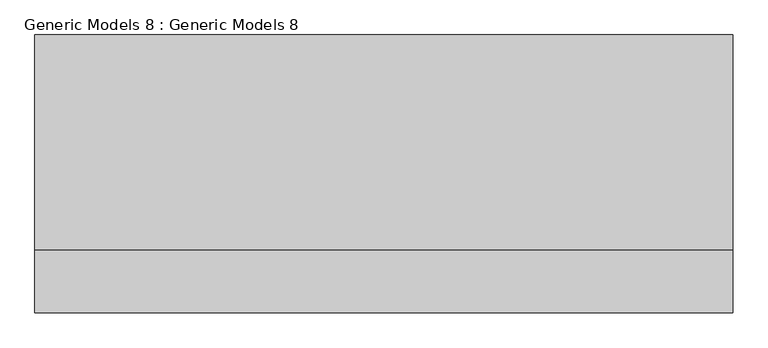
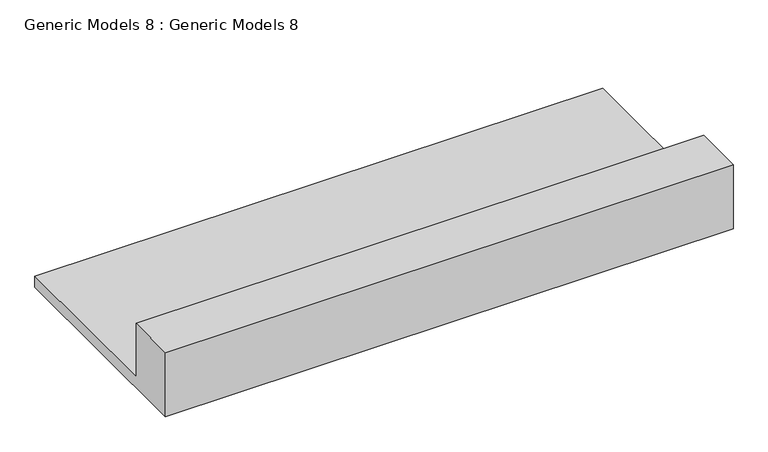
"""IFC4 building model written with IfcOpenShell, lengths in millimetres: proxy geometry, Generic Models 8 : Generic Models 8."""

from ifc_helpers import new_model, si_unit, frame, origin, place, context, project, spatial, polyline, outline, extrude, source, transform, mapped, element, save


def generic_models_8_generic_models_8_7572a94e(model_context):
    return source(origin(), model_context, "Body", "SweptSolid", [
        extrude(outline(polyline([(-3532.661407, 3657.6), (-3532.661407, 3962.4), (-3304.061407, 3962.4), (-3304.061407, 3708.4), (-2516.661407, 3708.4), (-2516.661407, 3657.6), (-3532.661407, 3657.6)])), frame((-14902.5371373, 0.0, 0.0), z_axis=(1.0, 0.0, 0.0), x_axis=(0.0, 1.0, 0.0)), (0.0, 0.0, 1.0), 2552.7),
    ])


if __name__ == "__main__":
    model = new_model("IFC4")
    model_context = context("Model", 3, world=origin())
    ifc_project = project(units=[si_unit("LENGTHUNIT", "METRE", prefix="MILLI")], contexts=[model_context])
    site = spatial("IfcSite", under=ifc_project)
    building = spatial("IfcBuilding", under=site)
    placement = place(None, origin())
    generic_models_8_generic_models_8_shape = generic_models_8_generic_models_8_7572a94e(model_context)
    element("IfcBuildingElementProxy", 1, Name="Generic Models 8 : Generic Models 8", ObjectType="Generic Models 8 : Generic Models 8", at=placement, inside=building, context=model_context, shape_type="MappedRepresentation", body=[
        mapped(generic_models_8_generic_models_8_shape, transform((0.0, 0.0, 0.0), x_axis=(1.0, 0.0, 0.0), y_axis=(0.0, 1.0, 0.0), z_axis=(0.0, 0.0, 1.0))),
    ])
    save(model, "model.ifc")

# Revit data of these elements
# Element 1 (IfcBuildingElementProxy, "Generic Models 8 : Generic Models 8")
#   Materials on its faces: "Gypsum Wall Board"
# Materials
#   "Gypsum Wall Board": class "Generic", colour RGB 127 127 127, transparency 0, Description = "Gypsum Wall Board", Cost = 0
